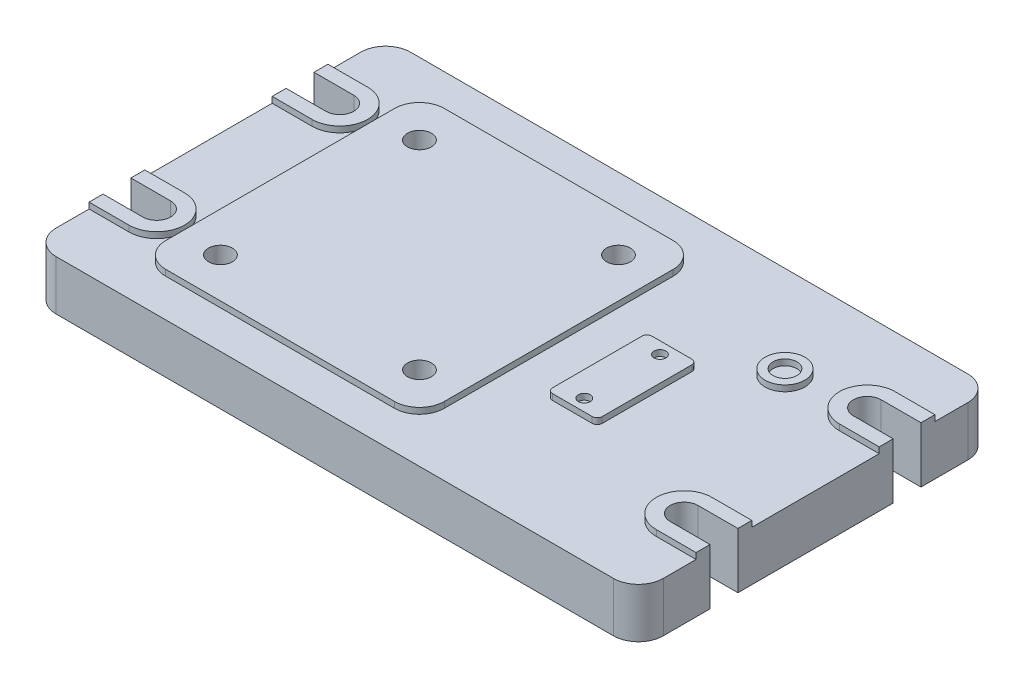
from build123d import *

# Parameters (mm, degrees)
BASE_PLATE_305X178X25_DEPTH        = 25
ROUND_BOSS_3MM_DEPTH               = 3
RAISED_PADS_SKETCH_R               = 10
RAISED_PADS_SKETCH_R_2             = 6
RAISED_PADS_SKETCH_R_3             = 3
RAISED_PADS_3MM_DEPTH              = 3
CORNER_FILLETS_R12_5_R             = 12.5
SLOT_RECESSES_10_DEEP_DEPTH        = 10
PAD_START                          = -18
PAD_HOLE_A_POSITION_SKETCH_R       = 7
PAD_HOLE_A_DEPTH                   = 10
PAD_HOLE_B_REACH                   = 180.332
PAD_HOLE_B_POSITION_SKETCH_R       = 6
PAD_HOLES_MIRROR_2_COPY_1_SKETCH_R = 7
PAD_HOLES_MIRROR_2_COPY_1_DEPTH    = 10
PAD_HOLES_MIRROR_2_COPY_2_REACH    = 180.332
PAD_HOLES_MIRROR_2_COPY_2_SKETCH_R = 6


with BuildPart() as part:
    # Base Plate Profile Sketch → Base Plate 305x178x25 (new body)
    with BuildSketch(Plane(origin=(0, 0, 0), x_dir=(1, 0, 0), z_dir=(0, 1, 0))):
        with BuildLine():
            Line((152.5, 89), (-152.5, 89))
            Line((-152.5, 89), (-152.5, 53))
            Line((-152.5, 53), (-132.5, 53))
            ThreePointArc((-132.5, 53), (-125.5, 46), (-132.5, 39))
            Line((-132.5, 39), (-152.5, 39))
            Line((-152.5, 39), (-152.5, -39))
            Line((-152.5, -39), (-132.5, -39))
            ThreePointArc((-132.5, -39), (-125.5, -46), (-132.5, -53))
            Line((-132.5, -53), (-152.5, -53))
            Line((-152.5, -53), (-152.5, -89))
            Line((-152.5, -89), (152.5, -89))
            Line((152.5, -89), (152.5, -53))
            Line((152.5, -53), (132.5, -53))
            ThreePointArc((132.5, -53), (125.5, -46), (132.5, -39))
            Line((132.5, -39), (152.5, -39))
            Line((152.5, -39), (152.5, 39))
            Line((152.5, 39), (132.5, 39))
            ThreePointArc((132.5, 39), (125.5, 46), (132.5, 53))
            Line((132.5, 53), (152.5, 53))
            Line((152.5, 53), (152.5, 89))
        make_face()
    extrude(amount=BASE_PLATE_305X178X25_DEPTH)

    # Round Boss Sketch → Round Boss 3mm (add)
    with BuildSketch(Plane(origin=(0, 25, 0), x_dir=(1, 0, 0), z_dir=(0, 1, 0))):
        with BuildLine():
            Line((-152.5, 60), (-152.5, 53))
            Line((-152.5, 53), (-132.5, 53))
            ThreePointArc((-132.5, 53), (-125.5, 46), (-132.5, 39))
            Line((-132.5, 39), (-152.5, 39))
            Line((-152.5, 39), (-152.5, 32))
            Line((-152.5, 32), (-132.5, 32))
            ThreePointArc((-132.5, 32), (-118.5, 46), (-132.5, 60))
            Line((-132.5, 60), (-152.5, 60))
        make_face()
        with BuildLine():
            Line((152.5, 53), (132.5, 53))
            ThreePointArc((132.5, 53), (125.5, 46), (132.5, 39))
            Line((132.5, 39), (152.5, 39))
            Line((152.5, 39), (152.5, 32))
            Line((152.5, 32), (132.5, 32))
            ThreePointArc((132.5, 32), (118.5, 46), (132.5, 60))
            Line((132.5, 60), (152.5, 60))
            Line((152.5, 60), (152.5, 53))
        make_face()
        with BuildLine():
            Line((152.5, -39), (132.5, -39))
            ThreePointArc((132.5, -39), (125.5, -46), (132.5, -53))
            Line((132.5, -53), (152.5, -53))
            Line((152.5, -53), (152.5, -60))
            Line((152.5, -60), (132.5, -60))
            ThreePointArc((132.5, -60), (118.5, -46), (132.5, -32))
            Line((132.5, -32), (152.5, -32))
            Line((152.5, -32), (152.5, -39))
        make_face()
        with BuildLine():
            Line((-152.5, -53), (-132.5, -53))
            ThreePointArc((-132.5, -53), (-125.5, -46), (-132.5, -39))
            Line((-132.5, -39), (-152.5, -39))
            Line((-152.5, -39), (-152.5, -32))
            Line((-152.5, -32), (-132.5, -32))
            ThreePointArc((-132.5, -32), (-118.5, -46), (-132.5, -60))
            Line((-132.5, -60), (-152.5, -60))
            Line((-152.5, -60), (-152.5, -53))
        make_face()
    extrude(amount=ROUND_BOSS_3MM_DEPTH)

    # Raised Pads Sketch → Raised Pads 3mm (add)
    # profile 1 of 3: a face of its own
    with BuildSketch(Plane(origin=(0, 25, 0), x_dir=(1, 0, 0), z_dir=(0, 1, 0))):
        with Locations(Location((94.809461238, 42.342376818, 0), (0, 0, 270))):
            Circle(RAISED_PADS_SKETCH_R)
        with Locations(Location((94.809461238, 42.342376818, 0), (0, 0, 270))):
            Circle(RAISED_PADS_SKETCH_R_2, mode=Mode.SUBTRACT)
    # profile 2 of 3: a face of its own
    with BuildSketch(Plane(origin=(0, 25, 0), x_dir=(1, 0, 0), z_dir=(0, 1, 0))):
        with BuildLine():
            Line((-104, 70), (11, 70))
            ThreePointArc((11, 70), (19.838834765, 66.338834765), (23.5, 57.5))
            Line((23.5, 57.5), (23.5, -57.5))
            ThreePointArc((23.5, -57.5), (19.838834765, -66.338834765), (11, -70))
            Line((11, -70), (-104, -70))
            ThreePointArc((-104, -70), (-112.838834765, -66.338834765), (-116.5, -57.5))
            Line((-116.5, -57.5), (-116.5, 57.5))
            ThreePointArc((-116.5, 57.5), (-112.838834765, 66.338834765), (-104, 70))
        make_face()
        with Locations(Location((-96.5, 50, 0), (0, 0, 270))):
            Circle(RAISED_PADS_SKETCH_R_2, mode=Mode.SUBTRACT)
        with Locations(Location((-96.5, -50, 0), (0, 0, 270))):
            Circle(RAISED_PADS_SKETCH_R_2, mode=Mode.SUBTRACT)
        with Locations(Location((3.5, -50, 0), (0, 0, 90))):
            Circle(RAISED_PADS_SKETCH_R_2, mode=Mode.SUBTRACT)
        with Locations(Location((3.5, 50, 0), (0, 0, 90))):
            Circle(RAISED_PADS_SKETCH_R_2, mode=Mode.SUBTRACT)
    # profile 3 of 3: a face of its own
    with BuildSketch(Plane(origin=(0, 25, 0), x_dir=(1, 0, 0), z_dir=(0, 1, 0))):
        with BuildLine():
            Line((47.228633365, 23.091650714), (67.228633365, 23.091650714))
            ThreePointArc((67.228633365, 23.091650714), (68.996400318, 22.359417667), (69.728633365, 20.591650714))
            Line((69.728633365, 20.591650714), (69.728633365, -24.408349286))
            ThreePointArc((69.728633365, -24.408349286), (68.996400318, -26.176116239), (67.228633365, -26.908349286))
            Line((67.228633365, -26.908349286), (47.228633365, -26.908349286))
            ThreePointArc((47.228633365, -26.908349286), (45.460866412, -26.176116239), (44.728633365, -24.408349286))
            Line((44.728633365, -24.408349286), (44.728633365, 20.591650714))
            ThreePointArc((44.728633365, 20.591650714), (45.460866412, 22.359417667), (47.228633365, 23.091650714))
        make_face()
        with Locations(Location((57.228633365, 17.091650714, 0), (0, 0, 270))):
            Circle(RAISED_PADS_SKETCH_R_3, mode=Mode.SUBTRACT)
        with Locations(Location((57.228633365, -20.908349286, 0), (0, 0, 270))):
            Circle(RAISED_PADS_SKETCH_R_3, mode=Mode.SUBTRACT)
    extrude(amount=RAISED_PADS_3MM_DEPTH)

    # Corner Fillets R12.5
    corner_fillets_r12_5_edges = [part.edges().sort_by_distance(p)[0] for p in [
        (-152.5, 12.5, -89),
        (152.5, 12.5, -89),
        (152.5, 12.5, 89),
        (-152.5, 12.5, 89),
    ]]
    fillet(corner_fillets_r12_5_edges, radius=CORNER_FILLETS_R12_5_R)

    # Slot Recess Sketch → Slot Recesses 10 Deep (cut)
    with BuildSketch(Plane.XZ):
        Polygon((-133.5, 25), (-133.5, -25), (-116.5, -25), (-116.5, -70), (116.5, -70), (116.5, -25), (133.5, -25), (133.5, 25), (116.5, 25), (116.5, 70), (-116.5, 70), (-116.5, 25), align=None)
    extrude(amount=-SLOT_RECESSES_10_DEEP_DEPTH, mode=Mode.SUBTRACT)

    # Pad Hole A Position Sketch → Pad Hole A (cut)
    with BuildSketch(Plane(origin=(0, 25, 0), x_dir=(1, 0, 0), z_dir=(0, 1, 0)).offset(PAD_START)):
        with Locations(Location((-96.5, -50, 0), (0, 0, 90))):
            Circle(PAD_HOLE_A_POSITION_SKETCH_R)
    pad_hole_a = extrude(amount=PAD_HOLE_A_DEPTH, mode=Mode.SUBTRACT)

    # Pad Hole B Position Sketch → Pad Hole B (cut, up to next)
    with BuildSketch(Plane(origin=(0, 25, 0), x_dir=(1, 0, 0), z_dir=(0, 1, 0)), mode=Mode.PRIVATE) as pad_hole_b_sk1:
        with Locations(Location((-96.5, -50, 0), (0, 0, 270))):
            Circle(PAD_HOLE_B_POSITION_SKETCH_R)
    pad_hole_b_tool1 = extrude(pad_hole_b_sk1.sketch, amount=-PAD_HOLE_B_REACH, mode=Mode.PRIVATE) & part.part
    pad_hole_b = pad_hole_b_tool1.solids().sort_by_distance((-96.5, 25, 50))[0]
    add(pad_hole_b, mode=Mode.SUBTRACT)

    # Pad Holes Mirror 1: Pad Hole A, Pad Hole B across plane
    add(pad_hole_a.mirror(Plane.ZY.offset(46.5)), mode=Mode.SUBTRACT)
    add(pad_hole_b.mirror(Plane.ZY.offset(46.5)), mode=Mode.SUBTRACT)

    # Pad Holes Mirror 2: Pad Hole A, Pad Hole B across plane
    add(pad_hole_a.mirror(Plane.XY), mode=Mode.SUBTRACT)
    add(pad_hole_b.mirror(Plane.XY), mode=Mode.SUBTRACT)

    # Pad Holes Mirror 2 copy 1 sketch → Pad Holes Mirror 2 copy 1 (cut)
    with BuildSketch(Plane(origin=(-93, 25, 0), x_dir=(-1, 0, 0), z_dir=(0, 1, 0)).offset(PAD_START)):
        with Locations(Location((-96.5, -50, 0), (0, 0, 90))):
            Circle(PAD_HOLES_MIRROR_2_COPY_1_SKETCH_R)
    extrude(amount=PAD_HOLES_MIRROR_2_COPY_1_DEPTH, mode=Mode.SUBTRACT)

    # Pad Holes Mirror 2 copy 2 sketch → Pad Holes Mirror 2 copy 2 (cut, up to next)
    with BuildSketch(Plane(origin=(-93, 25, 0), x_dir=(-1, 0, 0), z_dir=(0, 1, 0)), mode=Mode.PRIVATE) as pad_holes_mirror_2_copy_2_sk1:
        with Locations(Location((-96.5, -50, 0), (0, 0, 270))):
            Circle(PAD_HOLES_MIRROR_2_COPY_2_SKETCH_R)
    pad_holes_mirror_2_copy_2_tool1 = extrude(pad_holes_mirror_2_copy_2_sk1.sketch, amount=-PAD_HOLES_MIRROR_2_COPY_2_REACH, mode=Mode.PRIVATE) & part.part
    add(pad_holes_mirror_2_copy_2_tool1.solids().sort_by_distance((3.5, 25, -50))[0], mode=Mode.SUBTRACT)


solid = part.part
